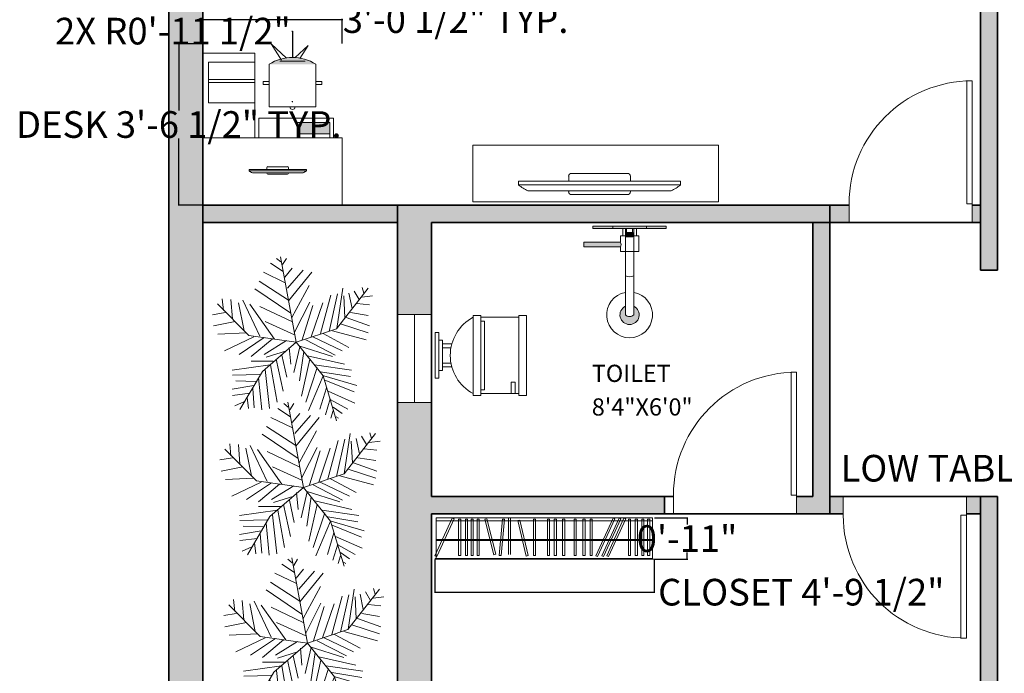
# Model space of a CAD drawing. Units: inches. Extents: x 1319 to 2030, y 219 to 1069.
# Tile 24 of 28: x 1331 to 1589, y 663 to 835. Entities that reach past the tile are written whole.
import ezdxf

# ---------------------------------------------------------------- set-up
doc = ezdxf.new("R2010")
doc.units = ezdxf.units.IN
doc.header["$MEASUREMENT"] = 0
doc.layers.get('0').update_dxf_attribs({"color": 12})
for name, color, linetype, lineweight in [('A-ANNO-DIMS', 2, 'Continuous', 18), ('A-AREA-IDEN', 250, 'Continuous', 18), ('A-GLAZ', 4, 'Continuous', 18), ('A-WALL-PATT', 252, 'Continuous', 13), ('C-PROP', 7, 'Continuous', 35), ('closet', 252, 'Continuous', 18), ('doors', 252, 'Continuous', 18), ('furniture', 250, 'Continuous', 18), ('lawn', 82, 'Continuous', 13), ('PLUMBING FIXTURES', 252, 'Continuous', 18), ('walls', 250, 'Continuous', 35)]:
    doc.layers.add(name, color=color, linetype=linetype, lineweight=lineweight)
doc.styles.get("Standard").update_dxf_attribs({"font": 'arial.ttf'})
doc.dimstyles.get("Standard").update_dxf_attribs({"dimtxt": 7, "dimasz": 0.18, "dimexe": 0.18, "dimexo": 0.0625, "dimgap": 0.09, "dimtad": 0, "dimtih": 1, "dimtoh": 1, "dimzin": 0, "dimdsep": 46, "dimlunit": 3, "dimtxsty": 'Standard', "dimcen": 0.09, "dimadec": 0, "dimazin": 0, "dimtfac": 1, "dimtofl": 0, "dimtmove": 0, "dimatfit": 3, "dimfxl": 1, "dimtolj": 1, "dimtzin": 0, "dimarcsym": 0})

# ---------------------------------------------------------------- blocks, each defined once
blk = doc.blocks.new('*U2')
for p, q in [((0, 0), (0, -6)), ((40, 0), (40, -6))]:
    blk.add_line(p, q)
blk.add_lwpolyline([(0, 0), (0, 40), (1.75, 40), (1.75, 0)], close=True)
blk.add_arc((0, 0), 40, 0, 90)
blk = doc.blocks.new('O.H SHOWER-PL')
at = {"layer": 'PLUMBING FIXTURES'}
for points in [[(-1.84, 0), (-1.84, -0.25), (1.84, -0.25), (1.84, 0)], [(0.46, -8.72), (0.46, -9.67, -0.422337), (-0.46, -9.67), (-0.46, -8.72, 4.325472)]]:
    blk.add_hatch(color=256, dxfattribs=at).paths.add_polyline_path(points)
for p, q in [((-1.84, 0), (-1.84, -0.25)), ((1.84, 0), (-1.84, 0)), ((1.84, 0), (1.84, -0.25)), ((1.84, -0.25), (-1.84, -0.25)), ((-0.46, -0.25), (-0.46, -9.67)), ((0.46, -0.25), (0.46, -9.67))]:
    blk.add_line(p, q, dxfattribs=at)
for centre, radius, start, end in [((0, -4.48), 1.03, 243.53, 296.47), ((0, -9.67), 2.5, 100.61, 79.39), ((0, -9.67), 1.05, 116.0349, 63.9652), ((0, -9.22), 0.643, 224.2078, 315.7922)]:
    blk.add_arc(centre, radius, start, end, dxfattribs=at)
blk = doc.blocks.new('DIVERTER-PL')
at = {"layer": 'PLUMBING FIXTURES'}
for points in [[(4, 0), (-4, 0), (-4, -0.25), (4, -0.25)], [(0.38, -1.14), (0.38, -0.7), (-0.37, -0.7), (-0.37, -1.14)], [(1, -1.75, 0.30818), (1, -2.25), (5, -2.25), (5, -1.75)]]:
    blk.add_hatch(color=256, dxfattribs=at).paths.add_polyline_path(points)
for p, q in [((-4, 0), (-4, -0.25)), ((-4, 0), (4, 0)), ((4, 0), (4, -0.25)), ((-4, -0.25), (4, -0.25)), ((-4, -0.25), (4, -0.25)), ((-1, -1.05), (-0.37, -1.05)), ((-1, -1.05), (-1, -2.75)), ((-0.75, -0.25), (-0.75, -1.05)), ((-0.37, -0.7), (0.38, -0.7)), ((-0.37, -0.7), (-0.37, -1.14)), ((-0.32, -0.7), (-0.32, -0.25)), ((0.32, -0.7), (0.32, -0.25)), ((0.38, -0.7), (0.38, -1.14)), ((0.38, -1.05), (1, -1.05)), ((0.75, -0.25), (0.75, -1.05)), ((1, -1.05), (1, -1.75)), ((-0.37, -1.14), (0.38, -1.14)), ((-1, -2.75), (1, -2.75)), ((1, -2.25), (1, -2.75))]:
    blk.add_line(p, q, dxfattribs=at)
at = {"layer": 'PLUMBING FIXTURES', "ltscale": 12}
for p, q in [((1, -1.75), (5, -1.75)), ((5, -2.25), (5, -1.75)), ((1, -2.25), (5, -2.25))]:
    blk.add_line(p, q, dxfattribs=at)
at = {"layer": 'PLUMBING FIXTURES'}
blk.add_arc((1.37, -2), 0.444, 145.7435, 214.2565, dxfattribs=at)
blk = doc.blocks.new('A$C7F153053')
at = {"layer": 'PLUMBING FIXTURES', "xscale": -1, "rotation": 270}
for name in ['DIVERTER-PL', 'O.H SHOWER-PL']:
    blk.add_blockref(name, (12.17, 4), dxfattribs=at)
blk = doc.blocks.new('*U25')
for p, q in [((-10, 22), (-10, 12)), ((-10, 21), (-7, 21)), ((-7, 21), (-7, 20)), ((10, 12), (10, 22)), ((-7, 20), (-10, 20)), ((9, 13), (-9, 13)), ((-9, 13), (-9, 12)), ((9, 12), (9, 13)), ((10.5, 12), (-10.5, 12)), ((-10.5, 10), (-10.5, 12)), ((10.5, 12), (10.5, 10)), ((10.5, 10), (-10.5, 10)), ((-3, 4.4065), (-3, 2)), ((-2, 2), (-2, 4.1658)), ((2, 4.1658), (2, 2)), ((3, 2), (3, 4.4065)), ((4, 2), (-4, 2)), ((-4, 2), (-4, 1)), ((4, 1), (4, 2))]:
    blk.add_line(p, q)
for points in [[(10.5, 22), (10.5, 24), (-10.5, 24), (-10.5, 22)], [(6, 0), (6, 1), (-6, 1), (-6, 0)]]:
    blk.add_lwpolyline(points, close=True)
blk.add_arc((0, 15.3333), 11.3333, 208.0725, 331.9275)
blk = doc.blocks.new('closet')
at = {"layer": 'closet'}
for p, q in [((-0.71, -5.58), (5.59, 8.19)), ((-0.23, 7.39), (-0.23, -6.57)), ((6.27, 7.88), (-0.04, -5.89)), ((5.59, 8.19), (6.27, 7.88)), ((7.92, 7.84), (8.68, 7.84)), ((7.92, 7.84), (7.92, -5.51)), ((8.68, 7.84), (8.68, -5.51)), ((10.44, 7.84), (11.2, 7.84)), ((10.44, 7.84), (10.44, -5.51)), ((11.2, 7.84), (11.2, -5.51)), ((12.45, 7.84), (13.21, 7.84)), ((12.45, 7.84), (12.45, -5.51)), ((13.21, 7.84), (13.21, -5.51)), ((14.71, 7.84), (15.47, 7.84)), ((14.71, 7.84), (14.71, -5.51)), ((15.47, 7.84), (15.47, -5.51)), ((17.44, 7.75), (18.17, 7.93)), ((17.44, 7.75), (20.73, -5.2)), ((18.17, 7.93), (21.46, -5.01)), ((23.92, 7.84), (22.75, -5.46)), ((24.67, 7.78), (23.51, -5.53)), ((23.92, 7.84), (24.67, 7.78)), ((26.09, 8.25), (26.09, -5.1)), ((26.84, 8.25), (26.84, -5.1)), ((29.49, 7.29), (32.64, -5.69)), ((30.22, 7.46), (33.37, -5.51)), ((35.23, 7.84), (35.23, -5.51)), ((35.99, 7.84), (35.99, -5.51)), ((40.33, 7.84), (40.33, -5.51)), ((41.08, 7.84), (41.08, -5.51)), ((42.85, 7.84), (42.85, -5.51)), ((43.61, 7.84), (43.61, -5.51)), ((45.9, 7.84), (45.9, -5.51)), ((46.65, 7.84), (46.65, -5.51)), ((50.07, 7.84), (50.07, -5.51)), ((50.82, 7.84), (50.82, -5.51)), ((53.32, 7.84), (53.32, -5.51)), ((54.08, 7.84), (54.08, -5.51)), ((55.9, 7.84), (55.9, -5.51)), ((56.65, 7.84), (56.65, -5.51)), ((57.99, -5.58), (64.3, 8.19)), ((64.97, 7.88), (58.67, -5.89)), ((60.19, -5.58), (66.49, 8.19)), ((67.17, 7.88), (60.87, -5.89)), ((62, -5.58), (68.3, 8.19)), ((68.98, 7.88), (62.67, -5.89)), ((69.96, 7.84), (69.96, -5.51)), ((70.72, 7.84), (70.72, -5.51)), ((72.43, 7.84), (72.43, -5.51)), ((73.19, 7.84), (73.19, -5.51)), ((74.82, 7.84), (74.82, -5.51)), ((75.57, 7.84), (75.57, -5.51)), ((76.94, 7.84), (76.94, -5.51)), ((77.69, 7.84), (77.69, -5.51)), ((56.23, 0.33), (0, 0.33)), ((56.2, 0), (0, 0)), ((56.2, 0), (78.76, 0)), ((56.23, 0.33), (78.76, 0.33)), ((-0.04, -5.89), (-0.71, -5.58)), ((21.46, -5.01), (20.73, -5.2)), ((23.51, -5.53), (22.75, -5.46)), ((33.37, -5.51), (32.64, -5.69)), ((35.99, -5.51), (35.23, -5.51)), ((41.08, -5.51), (40.33, -5.51)), ((43.61, -5.51), (42.85, -5.51)), ((46.65, -5.51), (45.9, -5.51)), ((50.82, -5.51), (50.07, -5.51)), ((54.08, -5.51), (53.32, -5.51)), ((56.65, -5.51), (55.9, -5.51)), ((58.67, -5.89), (57.99, -5.58)), ((60.87, -5.89), (60.19, -5.58)), ((62.67, -5.89), (62, -5.58)), ((70.72, -5.51), (69.96, -5.51)), ((73.19, -5.51), (72.43, -5.51)), ((75.57, -5.51), (74.82, -5.51)), ((77.69, -5.51), (76.94, -5.51))]:
    blk.add_line(p, q, dxfattribs=at)
blk = doc.blocks.new('rotated closet')
at = {"layer": 'closet'}
for p, q in [((26.32, 0.86), (27.07, 0.86)), ((29.72, -0.11), (30.45, 0.07)), ((35.46, 0.45), (36.22, 0.45)), ((40.56, 0.45), (41.31, 0.45)), ((43.08, 0.45), (43.84, 0.45)), ((46.13, 0.45), (46.88, 0.45)), ((50.3, 0.45), (51.05, 0.45)), ((53.56, 0.45), (54.31, 0.45)), ((56.13, 0.45), (56.88, 0.45)), ((64.53, 0.8), (65.2, 0.49)), ((66.72, 0.8), (67.4, 0.49)), ((68.53, 0.8), (69.21, 0.49)), ((70.19, 0.45), (70.95, 0.45)), ((72.66, 0.45), (73.42, 0.45)), ((75.05, 0.45), (75.81, 0.45)), ((77.17, 0.45), (77.92, 0.45)), ((78.99, 0), (78.99, -13.96)), ((-0.46, -14.27), (79.54, -14.27)), ((0, -13.96), (78.99, -13.96)), ((8.91, -12.91), (8.15, -12.91)), ((11.43, -12.91), (10.67, -12.91)), ((13.44, -12.91), (12.68, -12.91)), ((15.7, -12.91), (14.94, -12.91))]:
    blk.add_line(p, q, dxfattribs=at)
blk.add_blockref('closet', (0.23, -7.39), dxfattribs=at)
blk = doc.blocks.new('*U27')
for p, q in [((-8.737, 47.138), (-17.069, 52.711)), ((-10.186, 53.64), (-13.084, 55.962)), ((0, 0), (-10.5, 57)), ((-9.099, 51.782), (-6.563, 55.962)), ((-7.288, 39.707), (-21.778, 46.673)), ((-7.65, 43.423), (-2.578, 49.46)), ((-5.839, 35.992), (4.667, 48.067)), ((-5.114, 27.632), (10.463, 46.673)), ((-5.114, 28.097), (-24.676, 40.636)), ((-3.665, 19.273), (-27.574, 35.527)), ((-2.941, 16.486), (8.652, 37.85)), ((27, 9), (48, 36)), ((27.127, 9.056), (31.112, 35.992)), ((38.719, 34.134), (41.979, 28.561)), ((44.153, 36.456), (45.239, 32.741)), ((-48.585, 21.131), (-49.309, 29.026)), ((-43.513, 28.561), (-42.427, 15.558)), ((-35.544, 28.097), (-24.314, 3.947)), ((-1.129, 6.734), (9.014, 26.704)), ((16.259, 5.805), (23.142, 31.348)), ((22.055, 7.198), (27.489, 32.277)), ((31.836, 30.883), (32.561, 16.486)), ((35.096, 32.741), (37.27, 22.524)), ((43.791, 29.954), (51.036, 30.883)), ((-47.498, 19.737), (-55.83, 18.344)), ((-31.5, 4.5), (-52.5, 25.5)), ((-38.442, 26.239), (-34.819, 7.663)), ((-14.533, 2.09), (-30.834, 25.31)), ((-24.314, 23.917), (-2.941, 13.7)), ((3.942, 1.625), (11.187, 24.381)), ((10.101, 3.483), (17.708, 26.239)), ((36.183, 19.737), (48.137, 17.88)), ((40.53, 25.775), (48.862, 24.846)), ((-40.615, 13.7), (-55.105, 10.913)), ((-20.691, 13.7), (-1.129, 4.876)), ((33.285, 16.486), (48.862, 10.913)), ((0, 0), (27, 9)), ((24.229, 7.663), (46.688, 1.625)), ((29.662, 12.307), (48.137, 6.269)), ((-33.37, 6.269), (-52.207, 5.34)), ((-28.299, 3.483), (-47.86, -5.805)), ((-21.416, 3.018), (-38.079, -8.128)), ((0, 0), (-31.5, 4.5)), ((-15.982, 2.09), (-30.11, -9.521)), ((0, 0), (-22.5, -19.5)), ((-6.563, 1.161), (-21.416, -8.128)), ((0, 0), (18, -22.5)), ((6.478, 1.625), (26.04, -8.592)), ((11.187, 3.483), (30.749, -5.805)), ((18.07, 5.805), (35.096, -3.483)), ((-6.563, -5.805), (-19.967, -9.985)), ((-4.752, -3.483), (-3.665, -14.629)), ((2.493, -3.019), (-1.491, -20.202)), ((1.769, -2.555), (24.229, -9.521)), ((5.029, -6.27), (2.131, -25.775)), ((-15.257, -12.772), (-30.11, -12.772)), ((-13.446, -11.378), (-8.737, -32.741)), ((-9.461, -8.592), (-6.201, -23.453)), ((9.014, -11.378), (3.58, -35.992)), ((7.565, -9.056), (32.198, -14.629)), ((-17.431, -15.094), (-42.789, -18.809)), ((-22.5, -19.5), (-37.5, -45)), ((-20.691, -18.345), (-17.793, -44.352)), ((-17.069, -15.094), (-12.721, -40.172)), ((14.085, -16.951), (6.478, -40.172)), ((12.274, -15.094), (36.907, -18.809)), ((-24.314, -21.596), (-42.427, -22.06)), ((-26.849, -26.24), (-40.253, -25.775)), ((-25.038, -23.918), (-22.865, -45.281)), ((18.07, -22.524), (8.289, -45.745)), ((16.259, -19.738), (36.183, -22.989)), ((18, -22.5), (27, -52.5)), ((18.433, -22.524), (40.53, -29.026)), ((19.157, -25.311), (38.719, -33.206)), ((-28.299, -29.026), (-42.789, -31.348)), ((-29.023, -30.884), (-27.936, -43.887)), ((20.244, -30.419), (15.897, -44.816)), ((21.331, -32.741), (39.081, -40.636)), ((-30.834, -34.135), (-42.427, -35.528)), ((-32.646, -36.921), (-31.921, -44.352)), ((22.78, -37.85), (19.519, -48.532)), ((22.78, -38.314), (34.372, -44.816)), ((-34.457, -39.708), (-40.978, -42.494)), ((24.591, -45.745), (23.142, -50.854)), ((24.591, -43.423), (30.749, -47.603)), ((26.764, -49.925), (28.213, -50.854))]:
    blk.add_line(p, q)
blk = doc.blocks.new('PLASMA-LARGE')
at = {"layer": 'furniture'}
for p, q in [((-7.26, 0), (7.26, 0)), ((-21, -2.5), (21, -2.5)), ((-21, -2.5), (-21, -3.5)), ((-18.61, -1), (18.61, -1)), ((-8, -1), (-8, -0.74)), ((8, -1), (8, -0.74)), ((21, -2.5), (21, -3.5)), ((-21, -3.5), (21, -3.5)), ((-8, -3.5), (-8, -4.76)), ((8, -3.5), (8, -4.76)), ((-7.26, -5.5), (7.26, -5.5))]:
    blk.add_line(p, q, dxfattribs=at)
for centre, radius, start, end in [((-7.26, -0.74), 0.744, 90, 180), ((7.26, -0.74), 0.744, 0, 90), ((-13.97, -11.05), 11.07, 114.7602, 129.4175), ((13.97, -11.05), 11.07, 50.5825, 65.2398), ((-7.26, -4.76), 0.744, 180, 270), ((7.26, -4.76), 0.744, 270, 0)]:
    blk.add_arc(centre, radius, start, end, dxfattribs=at)
blk = doc.blocks.new('STUDY-STATION')
h = blk.add_hatch(color=256)
h.dxf.hatch_style = 1
h.paths.add_polyline_path([(29.65, 37, 0.288578), (17.34, 37)])
h = blk.add_hatch(color=256)
h.dxf.hatch_style = 1
h.paths.add_polyline_path([(33.33, 21.74), (24.73, 21.74), (24.73, 18.77), (33.33, 18.77)])
for p, q in [((20.6, 38.07), (17.92, 42.38)), ((17.92, 42.38), (21.92, 38.58)), ((27.56, 41.97), (24.23, 38.82)), ((25.39, 38.48), (27.56, 41.97)), ((13.58, 39.93), (0, 39.93)), ((13.58, 17.73), (13.58, 39.93)), ((13.58, 37.53), (1.44, 37.53)), ((1.44, 37.53), (1.44, 26.9)), ((17.34, 37), (17.34, 25.83)), ((26.82, 37.82), (20.17, 37.82)), ((29.65, 25.83), (29.65, 37)), ((13.58, 32.99), (1.44, 32.99)), ((1.44, 32.99), (1.44, 32.21)), ((1.44, 32.21), (13.58, 32.21)), ((13.58, 26.9), (13.58, 32.99)), ((17.34, 32.49), (15.81, 32.49)), ((15.81, 32.49), (15.81, 31.73)), ((15.81, 31.73), (17.34, 31.73)), ((17.34, 32.49), (17.34, 32.49)), ((29.65, 32.49), (31.18, 32.49)), ((31.18, 31.73), (29.65, 31.73)), ((31.18, 32.49), (31.18, 31.73)), ((1.44, 26.9), (13.58, 26.9)), ((17.34, 25.83), (29.65, 25.83)), ((14.64, 17.73), (14.64, 22.88)), ((14.64, 22.88), (34.27, 22.88)), ((24.73, 17.73), (24.73, 21.74)), ((24.73, 21.74), (33.33, 21.74)), ((33.33, 21.74), (33.33, 17.73)), ((34.27, 22.88), (34.27, 17.73)), ((24.73, 18.77), (33.33, 18.77)), ((0, 17.73), (36.53, 17.73)), ((36.53, 17.73), (36.53, 0))]:
    blk.add_line(p, q)
for centre, radius, start, end in [((23.49, 27.23), 11.55, 57.806, 122.194), ((23.49, 25.83), 0.688, 180, 0)]:
    blk.add_arc(centre, radius, start, end)
at = {"xscale": -0.3577737849257557, "yscale": 0.3577737849257557, "zscale": 0.3577737849257557, "rotation": 180}
blk.add_blockref('PLASMA-LARGE', (19.61, 8.15), dxfattribs=at)
blk = doc.blocks.new('MEDIA-CONSOLE')
for p, q in [((64.44, 14.9), (0, 14.9)), ((0, 14.9), (0, 0)), ((64.44, 0), (64.44, 14.9)), ((0, 0), (64.44, 0))]:
    blk.add_line(p, q)
at = {"xscale": -1.011294184530666, "yscale": 1.011294184530666, "zscale": 1.011294184530666, "rotation": 180}
blk.add_blockref('PLASMA-LARGE', (33.26, 1.95), dxfattribs=at)
blk = doc.blocks.new('*D44')
at = {"layer": 'A-ANNO-DIMS', "color": 0, "lineweight": -2, "transparency": 16777216}
for p, q in [((1661.46, 721.8), (1661.46, 716.99)), ((1692.74, 721.8), (1692.74, 716.99)), ((1661.46, 717.17), (1661.28, 717.17)), ((1692.56, 717.17), (1661.64, 717.17))]:
    blk.add_line(p, q, dxfattribs=at)
at = {"layer": 'A-ANNO-DIMS', "color": 0, "transparency": 16777216}
for points in [[(1661.64, 717.2), (1661.64, 717.14), (1661.46, 717.17)], [(1692.56, 717.2), (1692.56, 717.14), (1692.74, 717.17)]]:
    blk.add_solid(points, dxfattribs=at)
at = {"layer": 'Defpoints', "color": 0, "transparency": 16777216}
for p in [(1661.46, 721.86), (1692.74, 721.86), (1661.46, 717.17)]:
    blk.add_point(p, dxfattribs=at)
at = {"layer": 'A-ANNO-DIMS', "color": 0, "transparency": 16777216, "insert": (1602.51, 717.17), "char_height": 7, "attachment_point": 5}
blk.add_mtext('\\A1;LOW TABLE 2\'-7 1/2" TYP.', dxfattribs=at)
blk = doc.blocks.new('*D46')
at = {"layer": 'A-ANNO-DIMS', "color": 0, "lineweight": -2, "transparency": 16777216}
for p, q in [((1378.78, 828.6), (1372.31, 828.6)), ((1372.49, 828.42), (1372.49, 811.13)), ((1372.49, 786.41), (1372.49, 803.7)), ((1378.78, 786.23), (1372.31, 786.23))]:
    blk.add_line(p, q, dxfattribs=at)
at = {"layer": 'A-ANNO-DIMS', "color": 0, "transparency": 16777216}
for points in [[(1372.46, 828.42), (1372.52, 828.42), (1372.49, 828.6)], [(1372.46, 786.41), (1372.52, 786.41), (1372.49, 786.23)]]:
    blk.add_solid(points, dxfattribs=at)
at = {"layer": 'Defpoints', "color": 0, "transparency": 16777216}
for p in [(1372.49, 828.6), (1378.84, 828.6), (1378.84, 786.23)]:
    blk.add_point(p, dxfattribs=at)
at = {"layer": 'A-ANNO-DIMS', "color": 0, "transparency": 16777216, "insert": (1372.49, 807.41), "char_height": 7, "attachment_point": 5}
blk.add_mtext('\\A1;DESK 3\'-6 1/2" TYP.', dxfattribs=at)
blk = doc.blocks.new('*D47')
at = {"layer": 'A-ANNO-DIMS', "color": 0, "lineweight": -2, "transparency": 16777216}
for p, q in [((1378.84, 828.66), (1378.84, 835.14)), ((1379.02, 834.96), (1415.19, 834.96)), ((1415.37, 828.66), (1415.37, 835.14)), ((1415.37, 834.96), (1415.55, 834.96))]:
    blk.add_line(p, q, dxfattribs=at)
at = {"layer": 'A-ANNO-DIMS', "color": 0, "transparency": 16777216}
for points in [[(1379.02, 834.99), (1379.02, 834.93), (1378.84, 834.96)], [(1415.19, 834.99), (1415.19, 834.93), (1415.37, 834.96)]]:
    blk.add_solid(points, dxfattribs=at)
at = {"layer": 'Defpoints', "color": 0, "transparency": 16777216}
for p in [(1415.37, 834.96), (1378.84, 828.6), (1415.37, 828.6)]:
    blk.add_point(p, dxfattribs=at)
at = {"layer": 'A-ANNO-DIMS', "color": 0, "transparency": 16777216, "insert": (1445.13, 834.96), "char_height": 7, "attachment_point": 5}
blk.add_mtext('\\A1;3\'-0 1/2" TYP.', dxfattribs=at)
blk = doc.blocks.new('*D62')
at = {"layer": 'A-ANNO-DIMS', "color": 0, "lineweight": -2, "transparency": 16777216}
for p, q in [((1439.72, 693.2), (1439.72, 684.45)), ((1497.23, 693.2), (1497.23, 684.45)), ((1439.9, 684.63), (1497.05, 684.63)), ((1497.23, 684.63), (1497.41, 684.63))]:
    blk.add_line(p, q, dxfattribs=at)
at = {"layer": 'A-ANNO-DIMS', "color": 0, "transparency": 16777216}
for points in [[(1439.9, 684.66), (1439.9, 684.6), (1439.72, 684.63)], [(1497.05, 684.66), (1497.05, 684.6), (1497.23, 684.63)]]:
    blk.add_solid(points, dxfattribs=at)
at = {"layer": 'Defpoints', "color": 0, "transparency": 16777216}
for p in [(1439.72, 693.26), (1497.23, 693.26), (1497.23, 684.63)]:
    blk.add_point(p, dxfattribs=at)
at = {"layer": 'A-ANNO-DIMS', "color": 0, "transparency": 16777216, "insert": (1535.84, 684.63), "char_height": 7, "attachment_point": 5}
blk.add_mtext('\\A1;CLOSET 4\'-9 1/2"', dxfattribs=at)
blk = doc.blocks.new('*D63')
at = {"layer": 'A-ANNO-DIMS', "color": 0, "lineweight": -2, "transparency": 16777216}
for p, q in [((1497.29, 704.13), (1506.04, 704.13)), ((1505.86, 703.95), (1505.86, 702.36)), ((1505.86, 693.44), (1505.86, 695.03)), ((1497.29, 693.26), (1506.04, 693.26))]:
    blk.add_line(p, q, dxfattribs=at)
at = {"layer": 'A-ANNO-DIMS', "color": 0, "transparency": 16777216}
for points in [[(1505.83, 703.95), (1505.89, 703.95), (1505.86, 704.13)], [(1505.83, 693.44), (1505.89, 693.44), (1505.86, 693.26)]]:
    blk.add_solid(points, dxfattribs=at)
at = {"layer": 'Defpoints', "color": 0, "transparency": 16777216}
for p in [(1497.23, 704.13), (1505.86, 704.13), (1497.23, 693.26)]:
    blk.add_point(p, dxfattribs=at)
at = {"layer": 'A-ANNO-DIMS', "color": 0, "transparency": 16777216, "insert": (1505.86, 698.7), "char_height": 7, "attachment_point": 5}
blk.add_mtext('\\A1;0\'-11"', dxfattribs=at)
blk = doc.blocks.new('*D72')
at = {"layer": 'A-ANNO-DIMS', "color": 0, "lineweight": -2, "transparency": 16777216}
for p, q in [((1402.16, 831.93), (1402.34, 831.93)), ((1402.34, 831.93), (1402.34, 825.19)), ((1402.25, 813.46), (1402.43, 813.46)), ((1402.34, 813.37), (1402.34, 813.55))]:
    blk.add_line(p, q, dxfattribs=at)
at = {"layer": 'A-ANNO-DIMS', "color": 0, "transparency": 16777216}
blk.add_solid([(1402.37, 825.19), (1402.31, 825.19), (1402.34, 825.01)], dxfattribs=at)
at = {"layer": 'Defpoints', "color": 0, "transparency": 16777216}
for p in [(1402.34, 825.01), (1402.34, 813.46)]:
    blk.add_point(p, dxfattribs=at)
at = {"layer": 'A-ANNO-DIMS', "color": 0, "transparency": 16777216, "insert": (1370.96, 831.93), "char_height": 7, "attachment_point": 5}
blk.add_mtext('\\A1;2X R0\'-11 1/2"', dxfattribs=at)

msp = doc.modelspace()

# ---------------------------------------------------------------- hatches: boundary and pattern name
at = {"layer": 'A-WALL-PATT'}
h = msp.add_hatch(color=256, dxfattribs=at)
h.dxf.hatch_style = 1
h.paths.add_polyline_path([(1378.843, 946.227), (1960.843, 946.227), (1960.843, 860.616), (1922.194, 860.616), (1922.194, 851.616), (1960.843, 851.616), (1960.843, 304.227), (1578.343, 304.227), (1578.343, 295.227), (1969.843, 295.227), (1969.843, 955.227), (1369.843, 955.227), (1369.843, 295.227), (1378.843, 295.227)])
h = msp.add_hatch(color=256, dxfattribs=at)
h.dxf.hatch_style = 1
h.paths.add_polyline_path([(1856.292, 860.616), (1812.343, 860.616), (1812.343, 851.616), (1812.343, 700.993), (1816.843, 700.993), (1816.843, 851.616), (1856.292, 851.616)])
h.paths.add_polyline_path([(1960.843, 663.616), (1812.343, 663.616), (1782.783, 663.616), (1782.783, 659.116), (1812.343, 659.116), (1960.843, 659.116)])
h.paths.add_polyline_path([(1857.424, 659.116), (1852.924, 659.116), (1852.924, 616.807), (1857.424, 616.807)])
h.paths.add_polyline_path([(1735.843, 661.727), (1731.843, 661.727), (1636.133, 661.727), (1636.133, 657.227), (1731.343, 657.227), (1731.343, 481.227), (1618.616, 481.227), (1618.616, 472.227), (1639.343, 472.227), (1639.343, 384.227), (1627.044, 384.227), (1627.044, 375.227), (1648.343, 375.227), (1648.343, 384.227), (1648.343, 472.227), (1750.706, 472.227), (1750.706, 481.227), (1735.843, 481.227), (1735.843, 657.727)])
h.paths.add_polyline_path([(1587.343, 481.227), (1578.343, 481.227), (1578.343, 375.227), (1597.622, 375.227), (1597.622, 384.227), (1587.343, 384.227)])
h.paths.add_polyline_path([(1769.593, 384.227), (1693.482, 384.227), (1693.482, 375.227), (1769.593, 375.227)])
h.paths.add_polyline_path([(1775.828, 481.227), (1765.831, 481.227), (1765.831, 472.227), (1775.828, 472.227)])
h.paths.add_polyline_path([(1824.625, 481.227), (1820.343, 481.227), (1820.343, 476.727), (1824.625, 476.727), (1824.625, 477.545)], flags=0)
h.paths.add_polyline_path([(1896.843, 481.227), (1852.26, 481.227), (1852.26, 476.727), (1892.343, 476.727), (1892.343, 384.227), (1881.742, 384.227), (1881.742, 375.227), (1913.435, 375.227), (1913.435, 384.227), (1896.843, 384.227)])
h.paths.add_polyline_path([(1960.843, 481.227), (1931.341, 481.227), (1931.341, 476.727), (1960.843, 476.727)])
h.paths.add_polyline_path([(1736.343, 918.227), (1731.843, 918.227), (1731.843, 890.227), (1582.843, 890.227), (1582.843, 781.727), (1582.843, 769.171), (1587.343, 769.171), (1587.343, 781.727), (1587.343, 885.727), (1731.843, 885.727), (1731.843, 851.616), (1736.343, 851.616), (1736.343, 890.227)])
h.paths.add_polyline_path([(1781.022, 860.616), (1773.021, 860.616, -0.0322281), (1773.289, 856.464), (1773.289, 851.616), (1781.022, 851.616)])
h.paths.add_polyline_path([(1587.343, 946.227), (1582.843, 946.227), (1582.843, 926.136), (1587.343, 926.136)])
h.paths.add_polyline_path([(1647.843, 946.227), (1643.343, 946.227), (1643.343, 926.136), (1647.843, 926.136)])
h.paths.add_polyline_path([(1543.343, 786.227), (1429.843, 786.227), (1429.843, 757.555), (1434.343, 757.555), (1438.843, 757.555), (1438.843, 781.727), (1543.343, 781.727)])
h.paths.add_polyline_path([(1543.343, 781.727), (1538.843, 781.727), (1538.843, 709.727), (1534.597, 709.727), (1534.597, 705.227), (1543.343, 705.227), (1543.343, 709.727)])
h.paths.add_polyline_path([(1499.955, 709.727), (1438.843, 709.727), (1438.843, 734.463), (1429.843, 734.463), (1429.843, 552.227), (1470.241, 552.227), (1470.241, 561.227), (1438.843, 561.227), (1438.843, 705.227), (1499.955, 705.227)])
h.paths.add_polyline_path([(1587.343, 709.727), (1582.843, 709.727), (1582.843, 561.227), (1543.433, 561.227), (1543.433, 552.227), (1587.343, 552.227)])
h.paths.add_polyline_path([(1546.835, 709.727), (1543.343, 709.727), (1543.343, 705.227), (1546.835, 705.227)])
h.paths.add_polyline_path([(1582.843, 709.727), (1579.15, 709.727), (1579.15, 705.227), (1582.843, 705.227)], flags=17)
h.paths.add_polyline_path([(1548.368, 786.227), (1543.343, 786.227), (1543.343, 781.727), (1548.368, 781.727)])
h.paths.add_polyline_path([(1582.843, 786.227), (1580.683, 786.227), (1580.683, 781.727), (1582.843, 781.727)])
h.paths.add_polyline_path([(1587.343, 892.402), (1582.843, 892.402), (1582.843, 890.227), (1587.343, 890.227)], flags=17)
h.paths.add_polyline_path([(1647.843, 892.402), (1643.343, 892.402), (1643.343, 890.227), (1647.843, 890.227)], flags=17)
h.paths.add_polyline_path([(1740.974, 856.464), (1740.974, 860.616), (1736.343, 860.616), (1736.343, 851.616), (1740.974, 851.616)])
h.paths.add_polyline_path([(1853.989, 384.227), (1820.343, 384.227), (1820.343, 402.924), (1815.843, 402.924), (1815.843, 375.227), (1853.989, 375.227)])
h.paths.add_polyline_path([(1892.343, 436.227), (1820.343, 436.227), (1820.343, 481.227), (1815.843, 481.227), (1815.843, 431.727), (1892.343, 431.727)])
h.paths.add_polyline_path([(1849.175, 481.227), (1824.625, 481.227), (1824.625, 477.545), (1825.699, 477.545), (1825.699, 453.018, 0.4014527), (1849.175, 477.545)], flags=0)
h.paths.add_polyline_path([(1960.843, 384.227), (1941.188, 384.227), (1941.188, 375.227), (1960.843, 375.227)])
h.paths.add_polyline_path([(1902.267, 481.227), (1896.843, 481.227), (1896.843, 476.727), (1902.267, 476.727), (1902.267, 477.44)], flags=0)
h = msp.add_hatch(color=256, dxfattribs=at)
h.dxf.hatch_style = 1
h.paths.add_polyline_path([(1429.843, 786.227), (1378.843, 786.227), (1378.843, 781.727), (1429.843, 781.727)])

# ---------------------------------------------------------------- linework, layer by layer
at = {"layer": 'A-GLAZ'}
for p, q in [((1429.843, 757.555), (1438.843, 757.555)), ((1429.843, 734.463), (1429.843, 757.555)), ((1429.843, 757.555), (1434.343, 757.555)), ((1434.343, 757.555), (1434.343, 734.463)), ((1438.843, 757.555), (1438.843, 734.463)), ((1438.843, 734.463), (1429.843, 734.463))]:
    msp.add_line(p, q, dxfattribs=at)
at = {"layer": 'C-PROP'}
msp.add_line((1369.843, 295.227), (1369.843, 955.227), dxfattribs=at)
at = {"layer": 'closet'}
for p, q in [((1496.743, 703.388), (1439.978, 703.388)), ((1440.066, 704.127), (1440.066, 693.484)), ((1440.066, 704.127), (1496.831, 704.127)), ((1496.831, 693.484), (1496.831, 704.127)), ((1439.738, 693.258), (1439.738, 693.484)), ((1439.738, 693.484), (1440.066, 693.484)), ((1439.738, 693.258), (1497.23, 693.258)), ((1439.738, 693.258), (1497.23, 693.258)), ((1439.738, 693.258), (1497.23, 693.258)), ((1440.066, 693.484), (1495.65, 693.484)), ((1440.066, 693.484), (1496.831, 693.484))]:
    msp.add_line(p, q, dxfattribs=at)
at = {"layer": 'furniture'}
msp.add_line((1378.843, 803.958), (1378.843, 803.958), dxfattribs=at)
at = {"layer": 'walls'}
for p, q in [((1378.843, 295.227), (1378.843, 946.227)), ((1582.843, 781.727), (1582.843, 946.227)), ((1587.343, 781.727), (1587.343, 885.727)), ((1378.843, 786.227), (1548.368, 786.227)), ((1429.843, 552.227), (1429.843, 786.227)), ((1543.343, 709.727), (1543.343, 786.227)), ((1580.683, 786.227), (1582.843, 786.227)), ((1378.843, 781.727), (1429.843, 781.727)), ((1438.843, 781.727), (1582.843, 781.727)), ((1438.843, 709.727), (1438.843, 781.727)), ((1538.843, 709.727), (1538.843, 781.727)), ((1582.843, 781.727), (1582.843, 769.171)), ((1587.343, 769.171), (1587.343, 781.727)), ((1582.843, 769.171), (1587.343, 769.171)), ((1438.843, 709.727), (1502.283, 709.727)), ((1499.955, 709.727), (1499.955, 705.227)), ((1534.597, 709.727), (1538.843, 709.727)), ((1543.343, 709.727), (1587.343, 709.727)), ((1543.343, 709.727), (1543.343, 705.227)), ((1582.843, 561.227), (1582.843, 709.727)), ((1587.343, 531.767), (1587.343, 709.727)), ((1438.843, 561.227), (1438.843, 705.227)), ((1438.843, 705.227), (1546.835, 705.227)), ((1579.15, 705.227), (1582.843, 705.227))]:
    msp.add_line(p, q, dxfattribs=at)

# ---------------------------------------------------------------- block references
at = {"layer": 'closet', "xscale": 0.7186446519438578, "yscale": 0.7186446519438578, "zscale": 0.7186446519438578}
msp.add_blockref('rotated closet', (1440.066, 703.516), dxfattribs=at)
at = {"layer": 'doors', "xscale": -0.8078659498341503, "yscale": 0.8078659498341503, "zscale": 0.8078659498341503}
for p in [(1580.683, 786.574), (1534.597, 710.074)]:
    msp.add_blockref('*U2', p, dxfattribs=at)
at = {"layer": 'doors', "xscale": 0.8078659498341503, "yscale": 0.8078659498341503, "zscale": 0.8078659498341503, "rotation": 180}
msp.add_blockref('*U2', (1579.15, 704.88), dxfattribs=at)
at = {"layer": 'furniture'}
for name, p in [('STUDY-STATION', (1378.843, 786.227)), ('MEDIA-CONSOLE', (1449.633, 787.071))]:
    msp.add_blockref(name, p, dxfattribs=at)
at = {"layer": 'lawn', "xscale": 0.39313680782538, "yscale": 0.39313680782538, "zscale": 0.39313680782538}
for p in [(1403.297, 750.269), (1405.237, 712.13), (1406.267, 671.257)]:
    msp.add_blockref('*U27', p, dxfattribs=at)
at = {"layer": 'PLUMBING FIXTURES', "xscale": 2.406230429091579, "yscale": 2.406230429091579, "zscale": 2.406230429091579, "rotation": 90.00000000000003}
msp.add_blockref('A$C7F153053', (1500.41, 751.422), dxfattribs=at)
at = {"layer": 'PLUMBING FIXTURES', "xscale": -1, "rotation": 270}
msp.add_blockref('*U25', (1439.726, 746.789), dxfattribs=at)

# ---------------------------------------------------------------- texts
at = {"layer": 'A-AREA-IDEN'}
for s, p in [('TOILET', (1480.864, 739.825)), ('8\'4"X6\'0"', (1480.864, 731.002))]:
    msp.add_text(s, height=4.5146, dxfattribs=at).set_placement(p)

# ---------------------------------------------------------------- dimensions: what is measured, and where the dimension line sits
at = {"layer": 'A-ANNO-DIMS'}
for base, p1, p2, text, picture, middle in [((1415.373, 834.958), (1378.843, 828.602), (1415.373, 828.602), '<> TYP.', '*D47', (1445.131, 834.958)), ((1497.23, 684.631), (1439.721, 693.258), (1497.23, 693.258), 'CLOSET <>', '*D62', (1535.84, 684.631))]:
    dim = msp.add_linear_dim(base=base, p1=p1, p2=p2, text=text, dimstyle='Standard', override={"dimdec": 1, "dimlfac": 1, "dimrnd": 0, "dimzin": 1, "dimdsep": 46, "dimlunit": 4, "dimfrac": 2}, dxfattribs=at)
    dim.commit()
    dim.dimension.update_dxf_attribs({"geometry": picture, "text_midpoint": middle})
dim = msp.add_radius_dim(center=(1402.336, 813.457), mpoint=(1402.336, 825.006), text='2X <>', dimstyle='Standard', override={"dimdec": 1, "dimlfac": 1, "dimrnd": 0, "dimzin": 1, "dimdsep": 46, "dimlunit": 4, "dimfrac": 2}, dxfattribs=at)
dim.commit()
dim.dimension.update_dxf_attribs({"geometry": '*D72', "text_midpoint": (1370.957, 831.935), "dimtype": 164})
for base, p1, p2, angle, text, picture, middle in [((1372.487, 828.602), (1378.843, 786.227), (1378.843, 828.602), 90, 'DESK <> TYP.', '*D46', (1372.487, 807.415)), ((1661.464, 717.166), (1692.742, 721.858), (1661.464, 721.858), 180, 'LOW TABLE <> TYP.', '*D44', (1602.515, 717.166))]:
    dim = msp.add_linear_dim(base=base, p1=p1, p2=p2, angle=angle, text=text, dimstyle='Standard', override={"dimdec": 1, "dimlfac": 1, "dimrnd": 0, "dimzin": 1, "dimdsep": 46, "dimlunit": 4, "dimfrac": 2}, dxfattribs=at)
    dim.commit()
    dim.dimension.update_dxf_attribs({"geometry": picture, "text_midpoint": middle})
dim = msp.add_linear_dim(base=(1505.856, 704.134), p1=(1497.23, 693.258), p2=(1497.23, 704.134), angle=90, dimstyle='Standard', override={"dimdec": 1, "dimlfac": 1, "dimrnd": 0, "dimzin": 1, "dimdsep": 46, "dimlunit": 4, "dimfrac": 2}, dxfattribs=at)
dim.commit()
dim.dimension.update_dxf_attribs({"geometry": '*D63', "text_midpoint": (1505.856, 698.696)})

doc.saveas('drawing.dxf')
